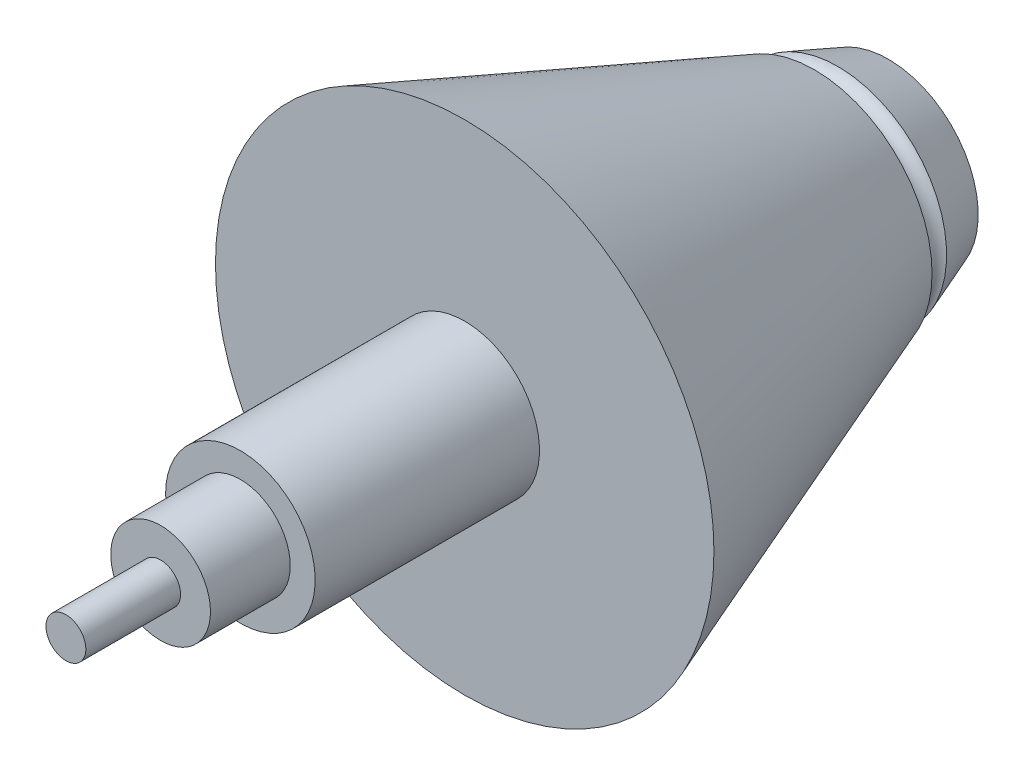
ISO-10303-21;
HEADER;
FILE_DESCRIPTION(('STEP AP214'),'2;1');
FILE_NAME('part.step','',(''),(''),'','','');
FILE_SCHEMA(('AUTOMOTIVE_DESIGN { 1 0 10303 214 1 1 1 1 }'));
ENDSEC;
DATA;
#1=APPLICATION_CONTEXT('core data for automotive mechanical design processes');
#2=APPLICATION_PROTOCOL_DEFINITION('international standard','automotive_design',2000,#1);
#3=PRODUCT_CONTEXT('',#1,'mechanical');
#4=PRODUCT('Part','Part','',(#3));
#5=PRODUCT_RELATED_PRODUCT_CATEGORY('part','',(#4));
#6=PRODUCT_DEFINITION_FORMATION('','',#4);
#7=PRODUCT_DEFINITION_CONTEXT('part definition',#1,'design');
#8=PRODUCT_DEFINITION('design','',#6,#7);
#9=PRODUCT_DEFINITION_SHAPE('','',#8);
#10=(LENGTH_UNIT() NAMED_UNIT(*) SI_UNIT(.MILLI.,.METRE.));
#11=(NAMED_UNIT(*) PLANE_ANGLE_UNIT() SI_UNIT($,.RADIAN.));
#12=(NAMED_UNIT(*) SI_UNIT($,.STERADIAN.) SOLID_ANGLE_UNIT());
#13=UNCERTAINTY_MEASURE_WITH_UNIT(LENGTH_MEASURE(1.E-05),#10,'distance_accuracy_value','');
#14=(GEOMETRIC_REPRESENTATION_CONTEXT(3) GLOBAL_UNCERTAINTY_ASSIGNED_CONTEXT((#13)) GLOBAL_UNIT_ASSIGNED_CONTEXT((#10,
#11,#12)) REPRESENTATION_CONTEXT('',''));
#15=CARTESIAN_POINT('',(0.,0.,0.));
#16=DIRECTION('',(0.,0.,1.));
#17=DIRECTION('',(1.,0.,0.));
#18=AXIS2_PLACEMENT_3D('',#15,#16,#17);
#19=CARTESIAN_POINT('',(0.,0.,45.));
#20=DIRECTION('',(0.,0.,-1.));
#21=DIRECTION('',(-1.,0.,0.));
#22=AXIS2_PLACEMENT_3D('',#19,#20,#21);
#23=CYLINDRICAL_SURFACE('',#22,15.);
#24=CARTESIAN_POINT('',(0.,0.,45.));
#25=DIRECTION('',(0.,0.,1.));
#26=DIRECTION('',(1.,0.,0.));
#27=AXIS2_PLACEMENT_3D('',#24,#25,#26);
#28=CIRCLE('',#27,15.);
#29=CARTESIAN_POINT('',(-15.,0.,45.));
#30=VERTEX_POINT('',#29);
#31=EDGE_CURVE('E131',#30,#30,#28,.T.);
#32=CARTESIAN_POINT('',(0.,0.,0.));
#33=DIRECTION('',(0.,0.,1.));
#34=DIRECTION('',(1.,0.,0.));
#35=AXIS2_PLACEMENT_3D('',#32,#33,#34);
#36=CIRCLE('',#35,15.);
#37=CARTESIAN_POINT('',(-15.,0.,0.));
#38=VERTEX_POINT('',#37);
#39=EDGE_CURVE('E145',#38,#38,#36,.T.);
#40=CARTESIAN_POINT('',(-15.,0.,45.));
#41=CARTESIAN_POINT('',(-15.,0.,44.53125));
#42=CARTESIAN_POINT('',(-15.,0.,44.0625));
#43=CARTESIAN_POINT('',(-15.,0.,43.125));
#44=CARTESIAN_POINT('',(-15.,0.,42.65625));
#45=CARTESIAN_POINT('',(-15.,0.,41.71875));
#46=CARTESIAN_POINT('',(-15.,0.,41.25));
#47=CARTESIAN_POINT('',(-15.,0.,40.3125));
#48=CARTESIAN_POINT('',(-15.,0.,39.84375));
#49=CARTESIAN_POINT('',(-15.,0.,38.90625));
#50=CARTESIAN_POINT('',(-15.,0.,38.4375));
#51=CARTESIAN_POINT('',(-15.,0.,37.5));
#52=CARTESIAN_POINT('',(-15.,0.,37.03125));
#53=CARTESIAN_POINT('',(-15.,0.,36.09375));
#54=CARTESIAN_POINT('',(-15.,0.,35.625));
#55=CARTESIAN_POINT('',(-15.,0.,34.6875));
#56=CARTESIAN_POINT('',(-15.,0.,34.21875));
#57=CARTESIAN_POINT('',(-15.,0.,33.28125));
#58=CARTESIAN_POINT('',(-15.,0.,32.8125));
#59=CARTESIAN_POINT('',(-15.,0.,31.875));
#60=CARTESIAN_POINT('',(-15.,0.,31.40625));
#61=CARTESIAN_POINT('',(-15.,0.,30.46875));
#62=CARTESIAN_POINT('',(-15.,0.,30.));
#63=CARTESIAN_POINT('',(-15.,0.,29.0625));
#64=CARTESIAN_POINT('',(-15.,0.,28.59375));
#65=CARTESIAN_POINT('',(-15.,0.,27.65625));
#66=CARTESIAN_POINT('',(-15.,0.,27.1875));
#67=CARTESIAN_POINT('',(-15.,0.,26.25));
#68=CARTESIAN_POINT('',(-15.,0.,25.78125));
#69=CARTESIAN_POINT('',(-15.,0.,24.84375));
#70=CARTESIAN_POINT('',(-15.,0.,24.375));
#71=CARTESIAN_POINT('',(-15.,0.,23.4375));
#72=CARTESIAN_POINT('',(-15.,0.,22.96875));
#73=CARTESIAN_POINT('',(-15.,0.,22.03125));
#74=CARTESIAN_POINT('',(-15.,0.,21.5625));
#75=CARTESIAN_POINT('',(-15.,0.,20.625));
#76=CARTESIAN_POINT('',(-15.,0.,20.15625));
#77=CARTESIAN_POINT('',(-15.,0.,19.21875));
#78=CARTESIAN_POINT('',(-15.,0.,18.75));
#79=CARTESIAN_POINT('',(-15.,0.,17.8125));
#80=CARTESIAN_POINT('',(-15.,0.,17.34375));
#81=CARTESIAN_POINT('',(-15.,0.,16.40625));
#82=CARTESIAN_POINT('',(-15.,0.,15.9375));
#83=CARTESIAN_POINT('',(-15.,0.,15.));
#84=CARTESIAN_POINT('',(-15.,0.,14.53125));
#85=CARTESIAN_POINT('',(-15.,0.,13.59375));
#86=CARTESIAN_POINT('',(-15.,0.,13.125));
#87=CARTESIAN_POINT('',(-15.,0.,12.1875));
#88=CARTESIAN_POINT('',(-15.,0.,11.71875));
#89=CARTESIAN_POINT('',(-15.,0.,10.78125));
#90=CARTESIAN_POINT('',(-15.,0.,10.3125));
#91=CARTESIAN_POINT('',(-15.,0.,9.37499999999999));
#92=CARTESIAN_POINT('',(-15.,0.,8.90624999999999));
#93=CARTESIAN_POINT('',(-15.,0.,7.96874999999999));
#94=CARTESIAN_POINT('',(-15.,0.,7.5));
#95=CARTESIAN_POINT('',(-15.,0.,6.56249999999999));
#96=CARTESIAN_POINT('',(-15.,0.,6.09374999999999));
#97=CARTESIAN_POINT('',(-15.,0.,5.15624999999999));
#98=CARTESIAN_POINT('',(-15.,0.,4.68749999999999));
#99=CARTESIAN_POINT('',(-15.,0.,3.74999999999999));
#100=CARTESIAN_POINT('',(-15.,0.,3.28124999999999));
#101=CARTESIAN_POINT('',(-15.,0.,2.34374999999999));
#102=CARTESIAN_POINT('',(-15.,0.,1.87499999999999));
#103=CARTESIAN_POINT('',(-15.,0.,0.937499999999992));
#104=CARTESIAN_POINT('',(-15.,0.,0.468749999999993));
#105=CARTESIAN_POINT('',(-15.,0.,0.));
#106=B_SPLINE_CURVE_WITH_KNOTS('',3,(#40,#41,#42,#43,#44,#45,#46,#47,#48,#49,#50,#51,#52,#53,
#54,#55,#56,#57,#58,#59,#60,#61,#62,#63,#64,#65,#66,#67,#68,#69,#70,#71,#72,#73,#74,#75,#76,#77,
#78,#79,#80,#81,#82,#83,#84,#85,#86,#87,#88,#89,#90,#91,#92,#93,#94,#95,#96,#97,#98,#99,#100,
#101,#102,#103,#104,#105),.UNSPECIFIED.,.F.,.F.,(4,2,2,2,2,2,2,2,2,2,2,2,2,2,2,2,2,2,2,2,2,2,2,
2,2,2,2,2,2,2,2,2,4),(0.,1.40625,2.8125,4.21874999999999,5.625,7.03125,8.43749999999999,9.84375,
11.25,12.65625,14.0625,15.46875,16.875,18.28125,19.6875,21.09375,22.5,23.90625,25.3125,26.71875,
28.125,29.53125,30.9375,32.34375,33.75,35.15625,36.5625,37.96875,39.375,40.78125,42.1875,
43.59375,45.),.UNSPECIFIED.);
#107=EDGE_CURVE('BSEAM54',#30,#38,#106,.T.);
#108=ORIENTED_EDGE('',*,*,#31,.F.);
#109=ORIENTED_EDGE('',*,*,#39,.T.);
#110=ORIENTED_EDGE('',*,*,#107,.T.);
#111=ORIENTED_EDGE('',*,*,#107,.F.);
#112=EDGE_LOOP('',(#108,#110,#109,#111));
#113=FACE_BOUND('',#112,.T.);
#114=ADVANCED_FACE('F54',(#113),#23,.T.);
#115=CARTESIAN_POINT('',(0.,0.,45.));
#116=DIRECTION('',(0.,0.,1.));
#117=DIRECTION('',(1.,0.,0.));
#118=AXIS2_PLACEMENT_3D('',#115,#116,#117);
#119=PLANE('',#118);
#120=CARTESIAN_POINT('',(0.,0.,45.));
#121=DIRECTION('',(0.,0.,1.));
#122=DIRECTION('',(1.,0.,0.));
#123=AXIS2_PLACEMENT_3D('',#120,#121,#122);
#124=CIRCLE('',#123,10.);
#125=CARTESIAN_POINT('',(10.,0.,45.));
#126=VERTEX_POINT('',#125);
#127=EDGE_CURVE('E128',#126,#126,#124,.T.);
#128=ORIENTED_EDGE('',*,*,#127,.F.);
#129=EDGE_LOOP('',(#128));
#130=FACE_BOUND('',#129,.T.);
#131=ORIENTED_EDGE('',*,*,#31,.T.);
#132=EDGE_LOOP('',(#131));
#133=FACE_BOUND('',#132,.T.);
#134=ADVANCED_FACE('F118',(#130,#133),#119,.T.);
#135=CARTESIAN_POINT('',(0.,0.,61.));
#136=DIRECTION('',(0.,0.,-1.));
#137=DIRECTION('',(-1.,0.,0.));
#138=AXIS2_PLACEMENT_3D('',#135,#136,#137);
#139=CYLINDRICAL_SURFACE('',#138,10.);
#140=CARTESIAN_POINT('',(0.,0.,61.));
#141=DIRECTION('',(0.,0.,1.));
#142=DIRECTION('',(1.,0.,0.));
#143=AXIS2_PLACEMENT_3D('',#140,#141,#142);
#144=CIRCLE('',#143,10.);
#145=CARTESIAN_POINT('',(10.,0.,61.));
#146=VERTEX_POINT('',#145);
#147=EDGE_CURVE('E134',#146,#146,#144,.T.);
#148=ORIENTED_EDGE('',*,*,#147,.F.);
#149=EDGE_LOOP('',(#148));
#150=FACE_BOUND('',#149,.T.);
#151=ORIENTED_EDGE('',*,*,#127,.T.);
#152=EDGE_LOOP('',(#151));
#153=FACE_BOUND('',#152,.T.);
#154=ADVANCED_FACE('F116',(#150,#153),#139,.T.);
#155=CARTESIAN_POINT('',(0.,0.,61.));
#156=DIRECTION('',(0.,0.,1.));
#157=DIRECTION('',(1.,0.,0.));
#158=AXIS2_PLACEMENT_3D('',#155,#156,#157);
#159=PLANE('',#158);
#160=CARTESIAN_POINT('',(0.,0.,61.));
#161=DIRECTION('',(0.,0.,1.));
#162=DIRECTION('',(1.,0.,0.));
#163=AXIS2_PLACEMENT_3D('',#160,#161,#162);
#164=CIRCLE('',#163,4.);
#165=CARTESIAN_POINT('',(4.,0.,61.));
#166=VERTEX_POINT('',#165);
#167=EDGE_CURVE('E137',#166,#166,#164,.T.);
#168=ORIENTED_EDGE('',*,*,#167,.F.);
#169=EDGE_LOOP('',(#168));
#170=FACE_BOUND('',#169,.T.);
#171=ORIENTED_EDGE('',*,*,#147,.T.);
#172=EDGE_LOOP('',(#171));
#173=FACE_BOUND('',#172,.T.);
#174=ADVANCED_FACE('F115',(#170,#173),#159,.T.);
#175=CARTESIAN_POINT('',(0.,0.,80.));
#176=DIRECTION('',(0.,0.,-1.));
#177=DIRECTION('',(-1.,0.,0.));
#178=AXIS2_PLACEMENT_3D('',#175,#176,#177);
#179=CYLINDRICAL_SURFACE('',#178,4.);
#180=CARTESIAN_POINT('',(0.,0.,80.));
#181=DIRECTION('',(0.,0.,1.));
#182=DIRECTION('',(1.,0.,0.));
#183=AXIS2_PLACEMENT_3D('',#180,#181,#182);
#184=CIRCLE('',#183,4.);
#185=CARTESIAN_POINT('',(4.,0.,80.));
#186=VERTEX_POINT('',#185);
#187=EDGE_CURVE('E136',#186,#186,#184,.T.);
#188=ORIENTED_EDGE('',*,*,#187,.F.);
#189=EDGE_LOOP('',(#188));
#190=FACE_BOUND('',#189,.T.);
#191=ORIENTED_EDGE('',*,*,#167,.T.);
#192=EDGE_LOOP('',(#191));
#193=FACE_BOUND('',#192,.T.);
#194=ADVANCED_FACE('F108',(#190,#193),#179,.T.);
#195=CARTESIAN_POINT('',(0.,0.,80.));
#196=DIRECTION('',(0.,0.,1.));
#197=DIRECTION('',(1.,0.,0.));
#198=AXIS2_PLACEMENT_3D('',#195,#196,#197);
#199=PLANE('',#198);
#200=ORIENTED_EDGE('',*,*,#187,.T.);
#201=EDGE_LOOP('',(#200));
#202=FACE_BOUND('',#201,.T.);
#203=ADVANCED_FACE('F104',(#202),#199,.T.);
#204=CARTESIAN_POINT('',(0.,0.,0.));
#205=DIRECTION('',(0.,0.,-1.));
#206=DIRECTION('',(-1.,0.,0.));
#207=AXIS2_PLACEMENT_3D('',#204,#205,#206);
#208=PLANE('',#207);
#209=ORIENTED_EDGE('',*,*,#39,.F.);
#210=EDGE_LOOP('',(#209));
#211=FACE_BOUND('',#210,.T.);
#212=CARTESIAN_POINT('',(0.,0.,0.));
#213=DIRECTION('',(0.,0.,-1.));
#214=DIRECTION('',(-1.,0.,0.));
#215=AXIS2_PLACEMENT_3D('',#212,#213,#214);
#216=CIRCLE('',#215,50.);
#217=CARTESIAN_POINT('',(-50.,0.,0.));
#218=VERTEX_POINT('',#217);
#219=EDGE_CURVE('E73',#218,#218,#216,.T.);
#220=ORIENTED_EDGE('',*,*,#219,.F.);
#221=EDGE_LOOP('',(#220));
#222=FACE_BOUND('',#221,.T.);
#223=ADVANCED_FACE('F98',(#211,#222),#208,.F.);
#224=CARTESIAN_POINT('',(0.,0.,-85.));
#225=DIRECTION('',(0.,0.,1.));
#226=DIRECTION('',(1.,0.,0.));
#227=AXIS2_PLACEMENT_3D('',#224,#225,#226);
#228=CONICAL_SURFACE('',#227,18.,0.360059329351052);
#229=CARTESIAN_POINT('',(0.,0.,-70.1711724782515));
#230=DIRECTION('',(0.,0.,-1.));
#231=DIRECTION('',(-1.,0.,0.));
#232=AXIS2_PLACEMENT_3D('',#229,#230,#231);
#233=CIRCLE('',#232,23.5826174199524);
#234=CARTESIAN_POINT('',(-23.5826174199526,0.,-70.1711724782515));
#235=VERTEX_POINT('',#234);
#236=EDGE_CURVE('E65',#235,#235,#233,.T.);
#237=ORIENTED_EDGE('',*,*,#236,.F.);
#238=EDGE_LOOP('',(#237));
#239=FACE_BOUND('',#238,.T.);
#240=ORIENTED_EDGE('',*,*,#219,.T.);
#241=EDGE_LOOP('',(#240));
#242=FACE_BOUND('',#241,.T.);
#243=ADVANCED_FACE('F88',(#239,#242),#228,.T.);
#244=CARTESIAN_POINT('',(0.,0.,-72.5));
#245=DIRECTION('',(0.,0.,-1.));
#246=DIRECTION('',(-1.,0.,0.));
#247=AXIS2_PLACEMENT_3D('',#244,#245,#246);
#248=TOROIDAL_SURFACE('',#247,22.6734626619789,2.5);
#249=CARTESIAN_POINT('',(0.,0.,-74.8502074609939));
#250=DIRECTION('',(0.,0.,1.));
#251=DIRECTION('',(1.,0.,0.));
#252=AXIS2_PLACEMENT_3D('',#249,#250,#251);
#253=CIRCLE('',#252,21.8210983676258);
#254=CARTESIAN_POINT('',(-21.8210983676256,0.,-74.8502074609939));
#255=VERTEX_POINT('',#254);
#256=EDGE_CURVE('E12',#255,#255,#253,.T.);
#257=ORIENTED_EDGE('',*,*,#256,.T.);
#258=CARTESIAN_POINT('',(-22.6734626619789,0.,-72.5));
#259=DIRECTION('',(0.,1.,0.));
#260=DIRECTION('',(0.,0.,1.));
#261=AXIS2_PLACEMENT_3D('',#258,#259,#260);
#262=CIRCLE('',#261,2.5);
#263=EDGE_CURVE('E66',#235,#255,#262,.T.);
#264=ORIENTED_EDGE('',*,*,#263,.F.);
#265=ORIENTED_EDGE('',*,*,#236,.T.);
#266=ORIENTED_EDGE('',*,*,#263,.T.);
#267=EDGE_LOOP('',(#257,#264,#265,#266));
#268=FACE_BOUND('',#267,.T.);
#269=ADVANCED_FACE('F69',(#268),#248,.F.);
#270=CARTESIAN_POINT('',(0.,0.,-85.));
#271=DIRECTION('',(0.,0.,-1.));
#272=DIRECTION('',(-1.,0.,0.));
#273=AXIS2_PLACEMENT_3D('',#270,#271,#272);
#274=PLANE('',#273);
#275=CARTESIAN_POINT('',(0.,0.,-85.));
#276=DIRECTION('',(0.,0.,-1.));
#277=DIRECTION('',(-1.,0.,0.));
#278=AXIS2_PLACEMENT_3D('',#275,#276,#277);
#279=CIRCLE('',#278,18.);
#280=CARTESIAN_POINT('',(-18.,0.,-85.));
#281=VERTEX_POINT('',#280);
#282=EDGE_CURVE('E75',#281,#281,#279,.T.);
#283=ORIENTED_EDGE('',*,*,#282,.T.);
#284=EDGE_LOOP('',(#283));
#285=FACE_BOUND('',#284,.T.);
#286=ADVANCED_FACE('F100',(#285),#274,.T.);
#287=ORIENTED_EDGE('',*,*,#256,.F.);
#288=EDGE_LOOP('',(#287));
#289=FACE_BOUND('',#288,.T.);
#290=ORIENTED_EDGE('',*,*,#282,.F.);
#291=EDGE_LOOP('',(#290));
#292=FACE_BOUND('',#291,.T.);
#293=ADVANCED_FACE('F96',(#289,#292),#228,.T.);
#294=CLOSED_SHELL('',(#114,#134,#154,#174,#194,#203,#223,#243,#269,#286,#293));
#295=MANIFOLD_SOLID_BREP('B2',#294);
#296=ADVANCED_BREP_SHAPE_REPRESENTATION('',(#18,#295),#14);
#297=SHAPE_DEFINITION_REPRESENTATION(#9,#296);
ENDSEC;
END-ISO-10303-21;
